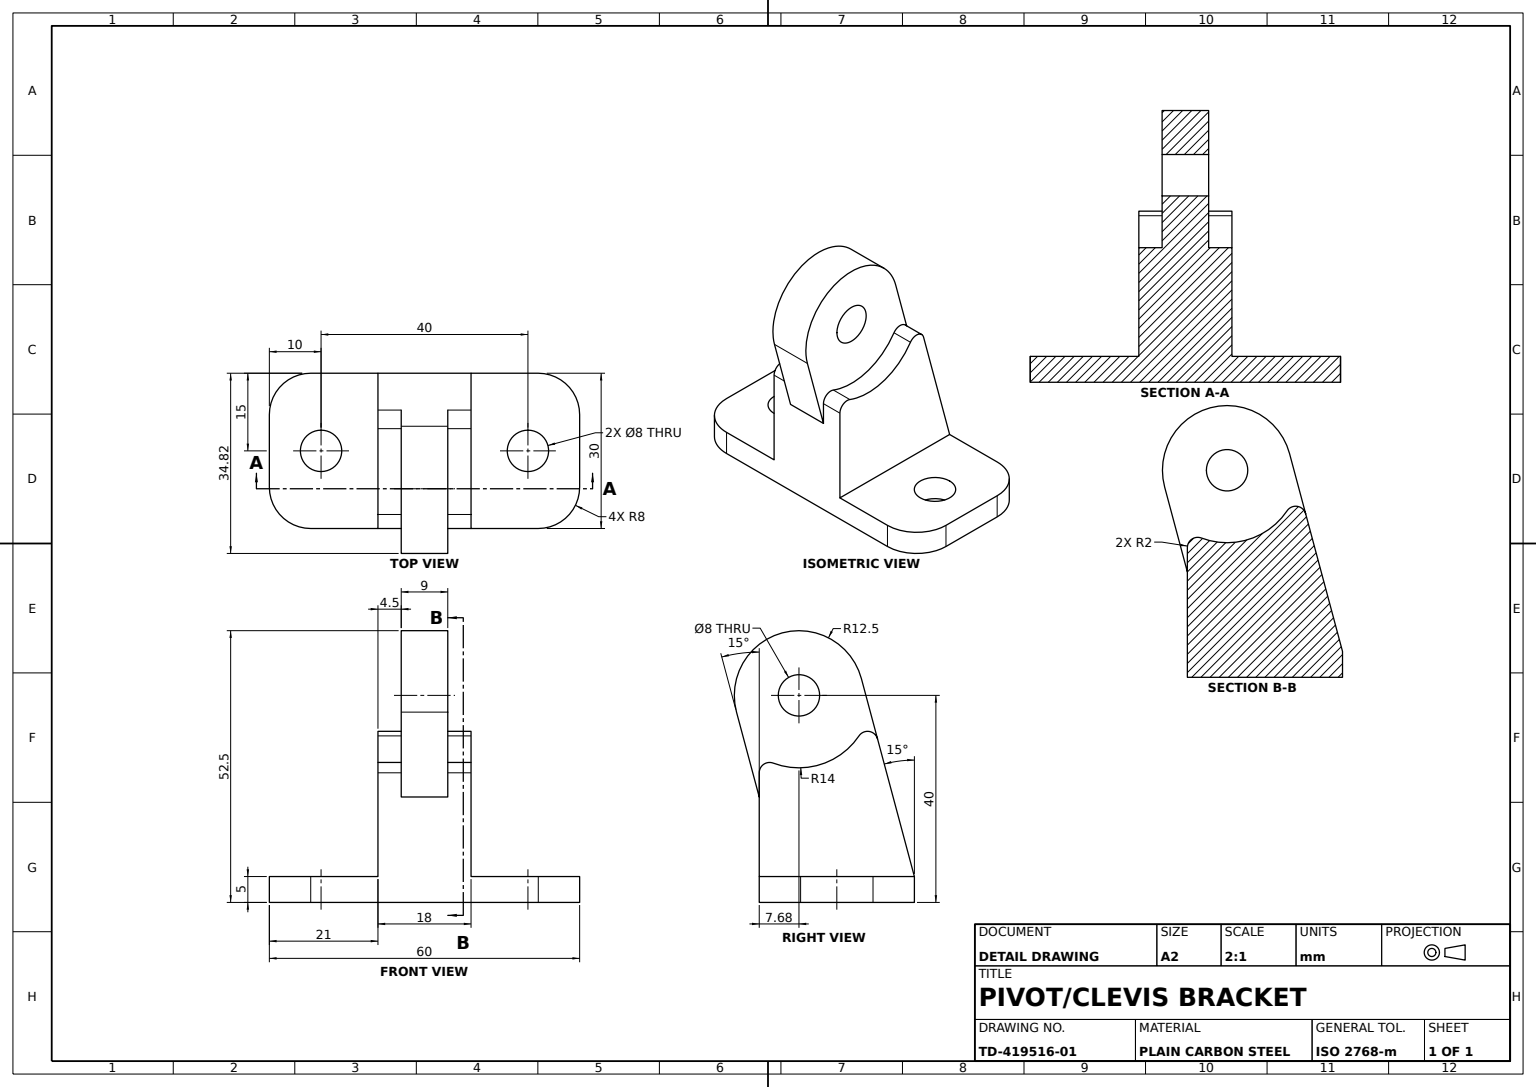
from build123d import *

# Parameters (mm, degrees)
BASE_PLATE_SKETCH_R       = 4
BASE_PLATE_DEPTH          = 5
TAPERED_UPRIGHT_DEPTH     = 9
PIVOT_LUG_DEPTH           = 10
LUG_SIDE_RELIEF_CUT_DEPTH = 5.5
PIVOT_BORE_SKETCH_R       = 4
PIVOT_BORE_8_DEPTH        = 66.873360759


with BuildPart() as part:
    # Base Plate Sketch → Base Plate (new body)
    with BuildSketch(Plane(origin=(0, 0, 0), x_dir=(1, 0, 0), z_dir=(0, 1, 0))):
        with BuildLine():
            Line((-22, 15), (22, 15))
            ThreePointArc((22, 15), (27.656854249, 12.656854249), (30, 7))
            Line((30, 7), (30, -7))
            ThreePointArc((30, -7), (27.656854249, -12.656854249), (22, -15))
            Line((22, -15), (-22, -15))
            ThreePointArc((-22, -15), (-27.656854249, -12.656854249), (-30, -7))
            Line((-30, -7), (-30, 7))
            ThreePointArc((-30, 7), (-27.656854249, 12.656854249), (-22, 15))
        make_face()
        with Locations(Location((-20, 0, 0), (0, 0, 270))):
            Circle(BASE_PLATE_SKETCH_R, mode=Mode.SUBTRACT)
        with Locations(Location((20, 0, 0), (0, 0, 270))):
            Circle(BASE_PLATE_SKETCH_R, mode=Mode.SUBTRACT)
    extrude(amount=BASE_PLATE_DEPTH)

    # Tapered Upright Sketch → Tapered Upright (add, symmetric)
    with BuildSketch(Plane(origin=(0, 0, 0), x_dir=(0, 0, -1), z_dir=(1, 0, 0))):
        with BuildLine():
            Line((-15, 20.368941598), (-15, 5))
            Line((-15, 5), (15, 5))
            Line((15, 5), (4.754898838, 43.235238064))
            ThreePointArc((4.754898838, 43.235238064), (-10.554412054, 52.074072829), (-19.393246819, 36.764761936))
            Line((-19.393246819, 36.764761936), (-15, 20.368941598))
        make_face()
    extrude(amount=TAPERED_UPRIGHT_DEPTH, both=True)

    # Pivot Lug Sketch → Pivot Lug (add, symmetric)
    with BuildSketch(Plane(origin=(0, 0, 0), x_dir=(0, 0, -1), z_dir=(1, 0, 0))):
        with BuildLine():
            Line((-15, 20.368941598), (-15, 25.04245288))
            ThreePointArc((-15, 25.04245288), (-14.135736214, 26.688692003), (-12.289896749, 26.91214627))
            ThreePointArc((-12.289896749, 26.91214627), (-3.083912061, 26.655991742), (4.289332839, 32.17423683))
            ThreePointArc((4.289332839, 32.17423683), (6.27753657, 33.028883618), (7.87954261, 31.573908753))
            Line((7.87954261, 31.573908753), (4.754898838, 43.235238064))
            ThreePointArc((4.754898838, 43.235238064), (-10.554412054, 52.074072829), (-19.393246819, 36.764761936))
            Line((-19.393246819, 36.764761936), (-15, 20.368941598))
        make_face()
    extrude(amount=PIVOT_LUG_DEPTH, both=True)

    # Lug Side Relief Sketch → Lug Side Relief Cut (cut)
    with BuildSketch(Plane(origin=(10, 0, 0), x_dir=(0, 0, -1), z_dir=(1, 0, 0))):
        with BuildLine():
            Line((-19.393246819, 36.764761936), (-15, 20.368941598))
            Line((-15, 20.368941598), (-15, 25.04245288))
            ThreePointArc((-15, 25.04245288), (-14.135736214, 26.688692003), (-12.289896749, 26.91214627))
            ThreePointArc((-12.289896749, 26.91214627), (-3.083912061, 26.655991742), (4.289332839, 32.17423683))
            ThreePointArc((4.289332839, 32.17423683), (6.27753657, 33.028883618), (7.87954261, 31.573908753))
            Line((7.87954261, 31.573908753), (4.754898838, 43.235238064))
            ThreePointArc((4.754898838, 43.235238064), (-10.554412054, 52.074072829), (-19.393246819, 36.764761936))
        make_face()
    lug_side_relief_cut = extrude(amount=-LUG_SIDE_RELIEF_CUT_DEPTH, mode=Mode.SUBTRACT)

    # Lug Side Relief Mirror: Lug Side Relief Cut across plane
    add(lug_side_relief_cut.mirror(Plane(origin=(0, 0, 0), x_dir=(0, 0, 1), z_dir=(1, 0, 0))), mode=Mode.SUBTRACT)

    # Pivot Bore Sketch → Pivot Bore Ø8 (cut, through all)
    with BuildSketch(Plane(origin=(4.5, 0, 0), x_dir=(0, 0, -1), z_dir=(1, 0, 0))):
        with Locations((-7.31917399, 40)):
            Circle(PIVOT_BORE_SKETCH_R)
    extrude(amount=-PIVOT_BORE_8_DEPTH, mode=Mode.SUBTRACT)


solid = part.part
